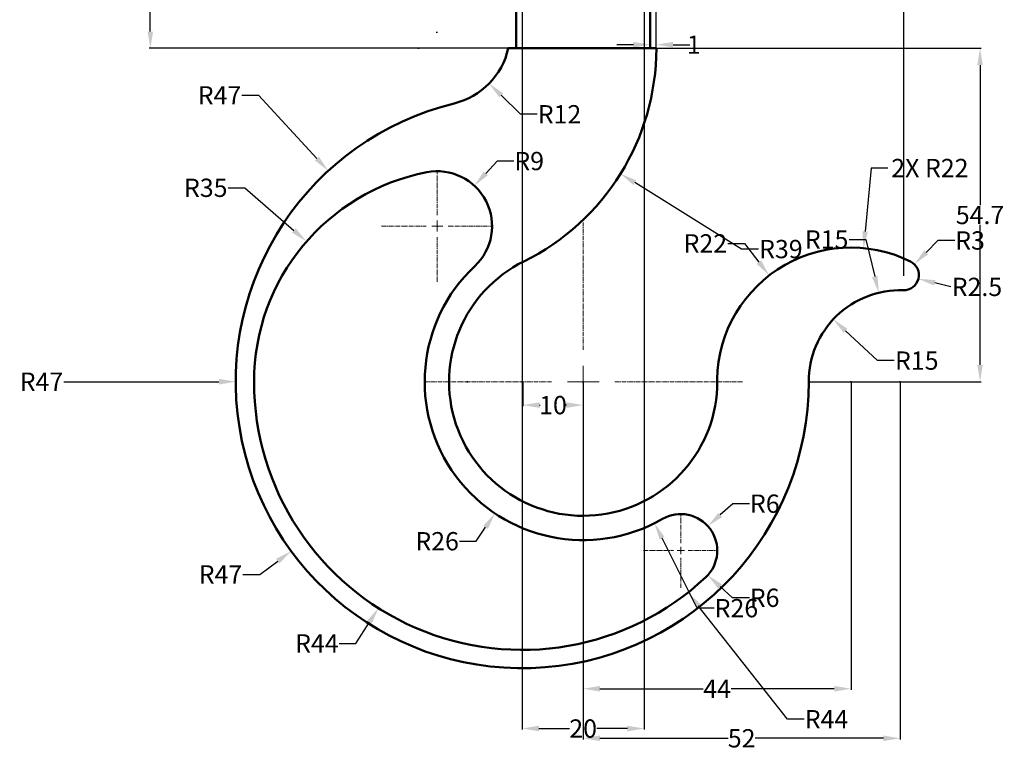
# Model space of a CAD drawing. Units: inches. Extents: x 7239 to 7401, y 3529 to 3727.
# Tile 1 of 2: x 7239 to 7400, y 3529 to 3648. Entities that reach past the tile are written whole.
import ezdxf

# ---------------------------------------------------------------- set-up
doc = ezdxf.new("R2010")
doc.units = ezdxf.units.IN
doc.header["$MEASUREMENT"] = 0
doc.linetypes.add('CENTER2', pattern=[1.125, 0.75, -0.125, 0.125, -0.125])
for name, color, linetype, lineweight in [('M-CNTR', 4, 'CENTER2', 18), ('M-DIMS', 2, 'Continuous', 25), ('M-OUTL', 7, 'Continuous', 50)]:
    doc.layers.add(name, color=color, linetype=linetype, lineweight=lineweight)
doc.styles.get("Standard").update_dxf_attribs({"font": 'arial.ttf'})
doc.dimstyles.get("Standard").update_dxf_attribs({"dimtxt": 3, "dimasz": 2.75, "dimexe": 0.18, "dimexo": 0.0625, "dimgap": 0.09, "dimtad": 0, "dimtih": 1, "dimtoh": 1, "dimdec": 0, "dimzin": 0, "dimdsep": 46, "dimtxsty": 'Standard', "dimcen": 0.09, "dimadec": 0, "dimazin": 0, "dimtfac": 1, "dimtdec": 0, "dimtofl": 0, "dimtmove": 0, "dimatfit": 3, "dimfxl": 1, "dimtolj": 1, "dimtzin": 0, "dimarcsym": 0})

# ---------------------------------------------------------------- blocks, each defined once
blk = doc.blocks.new('*U1')
at = {"layer": 'M-CNTR', "color": 0, "transparency": 16777216}
for p, q in [((0, 5.2), (0, 26.12)), ((-26.12, 0), (-5.2, 0)), ((5.2, 0), (26.12, 0)), ((0, -26.12), (0, -5.2))]:
    blk.add_line(p, q, dxfattribs=at)
at = {"layer": 'M-CNTR', "color": 0, "linetype": 'Continuous', "transparency": 16777216}
for p, q in [((0, -2.6), (0, 2.6)), ((-2.6, 0), (2.6, 0))]:
    blk.add_line(p, q, dxfattribs=at)
blk = doc.blocks.new('*U5')
at = {"layer": 'M-CNTR', "color": 0, "transparency": 16777216}
for p, q in [((0, 1.2), (0, 6.12)), ((-6.12, 0), (-1.2, 0)), ((1.2, 0), (6.12, 0)), ((0, -6.12), (0, -1.2))]:
    blk.add_line(p, q, dxfattribs=at)
at = {"layer": 'M-CNTR', "color": 0, "linetype": 'Continuous', "transparency": 16777216}
for p, q in [((-0.6, 0), (0.6, 0)), ((0, -0.6), (0, 0.6))]:
    blk.add_line(p, q, dxfattribs=at)
blk = doc.blocks.new('*U6')
at = {"layer": 'M-CNTR', "color": 0, "transparency": 16777216}
for p, q in [((0, 1.8), (0, 9.12)), ((-9.12, 0), (-1.8, 0)), ((1.8, 0), (9.12, 0)), ((0, -9.12), (0, -1.8))]:
    blk.add_line(p, q, dxfattribs=at)
at = {"layer": 'M-CNTR', "color": 0, "linetype": 'Continuous', "transparency": 16777216}
for p, q in [((-0.9, 0), (0.9, 0)), ((0, -0.9), (0, 0.9))]:
    blk.add_line(p, q, dxfattribs=at)
blk = doc.blocks.new('*D7')
at = {"layer": 'Defpoints', "color": 0, "transparency": 16777216}
for p in [(7289.29, 3623.58), (7321.11, 3589)]:
    blk.add_point(p, dxfattribs=at)
at = {"layer": 'M-DIMS', "color": 0, "lineweight": -2, "transparency": 16777216}
for p, q in [((7275.12, 3635.98), (7277.87, 3635.98)), ((7277.87, 3635.98), (7287.42, 3625.61)), ((7321.02, 3589), (7321.2, 3589)), ((7321.11, 3588.91), (7321.11, 3589.09))]:
    blk.add_line(p, q, dxfattribs=at)
at = {"layer": 'M-DIMS', "color": 0, "transparency": 16777216}
blk.add_solid([(7287.76, 3625.92), (7287.09, 3625.3), (7289.29, 3623.58)], dxfattribs=at)
at = {"layer": 'M-DIMS', "color": 0, "transparency": 16777216, "insert": (7271.45, 3635.98), "char_height": 3, "attachment_point": 5}
blk.add_mtext('\\A1;R47', dxfattribs=at)
blk = doc.blocks.new('*D8')
at = {"layer": 'Defpoints', "color": 0, "transparency": 16777216}
for p in [(7385.45, 3608.27), (7383.69, 3606.49)]:
    blk.add_point(p, dxfattribs=at)
at = {"layer": 'M-DIMS', "color": 0, "lineweight": -2, "transparency": 16777216}
for p, q in [((7389.32, 3612.17), (7387.38, 3610.22)), ((7392.07, 3612.17), (7389.32, 3612.17)), ((7383.6, 3606.49), (7383.78, 3606.49)), ((7383.69, 3606.4), (7383.69, 3606.58))]:
    blk.add_line(p, q, dxfattribs=at)
at = {"layer": 'M-DIMS', "color": 0, "transparency": 16777216}
blk.add_solid([(7387.06, 3610.54), (7387.71, 3609.9), (7385.45, 3608.27)], dxfattribs=at)
at = {"layer": 'M-DIMS', "color": 0, "transparency": 16777216, "insert": (7394.58, 3612.17), "char_height": 3, "attachment_point": 5}
blk.add_mtext('\\A1;R3', dxfattribs=at)
blk = doc.blocks.new('*D9')
at = {"layer": 'Defpoints', "color": 0, "transparency": 16777216}
for p in [(7372.14, 3599.23), (7383.11, 3589)]:
    blk.add_point(p, dxfattribs=at)
at = {"layer": 'M-DIMS', "color": 0, "lineweight": -2, "transparency": 16777216}
for p, q in [((7379.4, 3592.46), (7374.16, 3597.36)), ((7382.15, 3592.46), (7379.4, 3592.46))]:
    blk.add_line(p, q, dxfattribs=at)
at = {"layer": 'M-DIMS', "color": 0, "transparency": 16777216}
blk.add_solid([(7374.47, 3597.69), (7373.84, 3597.02), (7372.14, 3599.23)], dxfattribs=at)
at = {"layer": 'M-DIMS', "color": 0, "transparency": 16777216, "insert": (7385.84, 3592.46), "char_height": 3, "attachment_point": 5}
blk.add_mtext('\\A1;R15', dxfattribs=at)
blk = doc.blocks.new('*D10')
at = {"layer": 'Defpoints', "color": 0, "transparency": 16777216}
for p in [(7361.63, 3606.42), (7375.06, 3589)]:
    blk.add_point(p, dxfattribs=at)
at = {"layer": 'M-DIMS', "color": 0, "lineweight": -2, "transparency": 16777216}
for p, q in [((7354.82, 3611.69), (7357.57, 3611.69)), ((7357.57, 3611.69), (7359.95, 3608.6)), ((7374.97, 3589), (7375.15, 3589)), ((7375.06, 3588.91), (7375.06, 3589.09))]:
    blk.add_line(p, q, dxfattribs=at)
at = {"layer": 'M-DIMS', "color": 0, "transparency": 16777216}
blk.add_solid([(7360.31, 3608.88), (7359.59, 3608.32), (7361.63, 3606.42)], dxfattribs=at)
at = {"layer": 'M-DIMS', "color": 0, "transparency": 16777216, "insert": (7351.16, 3611.69), "char_height": 3, "attachment_point": 5}
blk.add_mtext('\\A1;R22', dxfattribs=at)
blk = doc.blocks.new('*D11')
at = {"layer": 'Defpoints', "color": 0, "transparency": 16777216}
for p in [(7351.57, 3565.31), (7347.11, 3561.29)]:
    blk.add_point(p, dxfattribs=at)
at = {"layer": 'M-DIMS', "color": 0, "lineweight": -2, "transparency": 16777216}
for p, q in [((7355.65, 3568.99), (7353.61, 3567.15)), ((7358.4, 3568.99), (7355.65, 3568.99)), ((7347.02, 3561.29), (7347.2, 3561.29)), ((7347.11, 3561.2), (7347.11, 3561.38))]:
    blk.add_line(p, q, dxfattribs=at)
at = {"layer": 'M-DIMS', "color": 0, "transparency": 16777216}
blk.add_solid([(7353.3, 3567.49), (7353.92, 3566.81), (7351.57, 3565.31)], dxfattribs=at)
at = {"layer": 'M-DIMS', "color": 0, "transparency": 16777216, "insert": (7360.91, 3568.99), "char_height": 3, "attachment_point": 5}
blk.add_mtext('\\A1;R6', dxfattribs=at)
blk = doc.blocks.new('*D12')
at = {"layer": 'Defpoints', "color": 0, "transparency": 16777216}
for p in [(7321.11, 3589), (7283.22, 3561.19)]:
    blk.add_point(p, dxfattribs=at)
at = {"layer": 'M-DIMS', "color": 0, "lineweight": -2, "transparency": 16777216}
for p, q in [((7321.02, 3589), (7321.2, 3589)), ((7321.11, 3588.91), (7321.11, 3589.09)), ((7278.04, 3557.39), (7281.01, 3559.57)), ((7275.29, 3557.39), (7278.04, 3557.39))]:
    blk.add_line(p, q, dxfattribs=at)
at = {"layer": 'M-DIMS', "color": 0, "transparency": 16777216}
blk.add_solid([(7280.74, 3559.94), (7281.28, 3559.2), (7283.22, 3561.19)], dxfattribs=at)
at = {"layer": 'M-DIMS', "color": 0, "transparency": 16777216, "insert": (7271.61, 3557.39), "char_height": 3, "attachment_point": 5}
blk.add_mtext('\\A1;R47', dxfattribs=at)
blk = doc.blocks.new('*D13')
at = {"layer": 'Defpoints', "color": 0, "transparency": 16777216}
for p in [(7321.11, 3589), (7297.52, 3551.86)]:
    blk.add_point(p, dxfattribs=at)
at = {"layer": 'M-DIMS', "color": 0, "lineweight": -2, "transparency": 16777216}
for p, q in [((7321.02, 3589), (7321.2, 3589)), ((7321.11, 3588.91), (7321.11, 3589.09)), ((7293.84, 3546.07), (7296.04, 3549.54)), ((7291.09, 3546.07), (7293.84, 3546.07))]:
    blk.add_line(p, q, dxfattribs=at)
at = {"layer": 'M-DIMS', "color": 0, "transparency": 16777216}
blk.add_solid([(7295.66, 3549.79), (7296.43, 3549.3), (7297.52, 3551.86)], dxfattribs=at)
at = {"layer": 'M-DIMS', "color": 0, "transparency": 16777216, "insert": (7287.42, 3546.07), "char_height": 3, "attachment_point": 5}
blk.add_mtext('\\A1;R44', dxfattribs=at)
blk = doc.blocks.new('*D14')
at = {"layer": 'Defpoints', "color": 0, "transparency": 16777216}
for p in [(7313.26, 3621.15), (7307.17, 3614.53)]:
    blk.add_point(p, dxfattribs=at)
at = {"layer": 'M-DIMS', "color": 0, "lineweight": -2, "transparency": 16777216}
for p, q in [((7316.99, 3625.2), (7315.12, 3623.17)), ((7319.74, 3625.2), (7316.99, 3625.2)), ((7307.08, 3614.53), (7307.26, 3614.53)), ((7307.17, 3614.44), (7307.17, 3614.62))]:
    blk.add_line(p, q, dxfattribs=at)
at = {"layer": 'M-DIMS', "color": 0, "transparency": 16777216}
blk.add_solid([(7314.79, 3623.48), (7315.46, 3622.86), (7313.26, 3621.15)], dxfattribs=at)
at = {"layer": 'M-DIMS', "color": 0, "transparency": 16777216, "insert": (7322.25, 3625.2), "char_height": 3, "attachment_point": 5}
blk.add_mtext('\\A1;R9', dxfattribs=at)
blk = doc.blocks.new('*D15')
at = {"layer": 'Defpoints', "color": 0, "transparency": 16777216}
for p in [(7331.11, 3589), (7316.64, 3567.4)]:
    blk.add_point(p, dxfattribs=at)
at = {"layer": 'M-DIMS', "color": 0, "lineweight": -2, "transparency": 16777216}
for p, q in [((7331.02, 3589), (7331.2, 3589)), ((7331.11, 3588.91), (7331.11, 3589.09)), ((7313.58, 3562.83), (7315.11, 3565.12)), ((7310.83, 3562.83), (7313.58, 3562.83))]:
    blk.add_line(p, q, dxfattribs=at)
at = {"layer": 'M-DIMS', "color": 0, "transparency": 16777216}
blk.add_solid([(7314.73, 3565.37), (7315.49, 3564.86), (7316.64, 3567.4)], dxfattribs=at)
at = {"layer": 'M-DIMS', "color": 0, "transparency": 16777216, "insert": (7307.15, 3562.83), "char_height": 3, "attachment_point": 5}
blk.add_mtext('\\A1;R26', dxfattribs=at)
blk = doc.blocks.new('*D16')
at = {"layer": 'Defpoints', "color": 0, "transparency": 16777216}
for p in [(7331.11, 3588.91), (7383.11, 3589), (7383.11, 3530.5)]:
    blk.add_point(p, dxfattribs=at)
at = {"layer": 'M-DIMS', "color": 0, "lineweight": -2, "transparency": 16777216}
for p, q in [((7331.11, 3588.85), (7331.11, 3530.32)), ((7383.11, 3588.94), (7383.11, 3530.32)), ((7333.86, 3530.5), (7354.89, 3530.5)), ((7380.36, 3530.5), (7359.34, 3530.5))]:
    blk.add_line(p, q, dxfattribs=at)
at = {"layer": 'M-DIMS', "color": 0, "transparency": 16777216}
for points in [[(7333.86, 3530.96), (7333.86, 3530.04), (7331.11, 3530.5)], [(7380.36, 3530.96), (7380.36, 3530.04), (7383.11, 3530.5)]]:
    blk.add_solid(points, dxfattribs=at)
at = {"layer": 'M-DIMS', "color": 0, "transparency": 16777216, "insert": (7357.11, 3530.5), "char_height": 3, "attachment_point": 5}
blk.add_mtext('\\A1;52', dxfattribs=at)
blk = doc.blocks.new('*D17')
at = {"layer": 'Defpoints', "color": 0, "transparency": 16777216}
for p in [(7331.11, 3588.91), (7375.06, 3588.91), (7375.06, 3538.63)]:
    blk.add_point(p, dxfattribs=at)
at = {"layer": 'M-DIMS', "color": 0, "lineweight": -2, "transparency": 16777216}
for p, q in [((7331.11, 3588.85), (7331.11, 3538.45)), ((7375.06, 3588.85), (7375.06, 3538.45)), ((7333.86, 3538.63), (7350.8, 3538.63)), ((7372.31, 3538.63), (7355.38, 3538.63))]:
    blk.add_line(p, q, dxfattribs=at)
at = {"layer": 'M-DIMS', "color": 0, "transparency": 16777216}
for points in [[(7333.86, 3539.09), (7333.86, 3538.17), (7331.11, 3538.63)], [(7372.31, 3539.09), (7372.31, 3538.17), (7375.06, 3538.63)]]:
    blk.add_solid(points, dxfattribs=at)
at = {"layer": 'M-DIMS', "color": 0, "transparency": 16777216, "insert": (7353.09, 3538.63), "char_height": 3, "attachment_point": 5}
blk.add_mtext('\\A1;44', dxfattribs=at)
blk = doc.blocks.new('*D18')
at = {"layer": 'Defpoints', "color": 0, "transparency": 16777216}
for p in [(7321.2, 3589), (7331.11, 3589.09), (7321.2, 3585.16)]:
    blk.add_point(p, dxfattribs=at)
at = {"layer": 'M-DIMS', "color": 0, "lineweight": -2, "transparency": 16777216}
for p, q in [((7321.2, 3588.94), (7321.2, 3584.98)), ((7331.11, 3589.03), (7331.11, 3584.98)), ((7323.95, 3585.16), (7324.07, 3585.16)), ((7328.36, 3585.16), (7328.25, 3585.16))]:
    blk.add_line(p, q, dxfattribs=at)
at = {"layer": 'M-DIMS', "color": 0, "transparency": 16777216}
for points in [[(7323.95, 3585.62), (7323.95, 3584.7), (7321.2, 3585.16)], [(7328.36, 3585.62), (7328.36, 3584.7), (7331.11, 3585.16)]]:
    blk.add_solid(points, dxfattribs=at)
at = {"layer": 'M-DIMS', "color": 0, "transparency": 16777216, "insert": (7326.16, 3585.16), "char_height": 3, "attachment_point": 5}
blk.add_mtext('\\A1;10', dxfattribs=at)
blk = doc.blocks.new('*D19')
at = {"layer": 'Defpoints', "color": 0, "transparency": 16777216}
for p in [(7285.73, 3612), (7312.11, 3589)]:
    blk.add_point(p, dxfattribs=at)
at = {"layer": 'M-DIMS', "color": 0, "lineweight": -2, "transparency": 16777216}
for p, q in [((7272.88, 3620.81), (7275.63, 3620.81)), ((7275.63, 3620.81), (7283.66, 3613.81)), ((7312.02, 3589), (7312.2, 3589)), ((7312.11, 3588.91), (7312.11, 3589.09))]:
    blk.add_line(p, q, dxfattribs=at)
at = {"layer": 'M-DIMS', "color": 0, "transparency": 16777216}
blk.add_solid([(7283.96, 3614.15), (7283.36, 3613.46), (7285.73, 3612)], dxfattribs=at)
at = {"layer": 'M-DIMS', "color": 0, "transparency": 16777216, "insert": (7269.19, 3620.81), "char_height": 3, "attachment_point": 5}
blk.add_mtext('\\A1;R35', dxfattribs=at)
blk = doc.blocks.new('*D20')
at = {"layer": 'Defpoints', "color": 0, "transparency": 16777216}
for p in [(7343.11, 3644.29), (7342.11, 3643.7), (7343.11, 3643.7)]:
    blk.add_point(p, dxfattribs=at)
at = {"layer": 'M-DIMS', "color": 0, "lineweight": -2, "transparency": 16777216}
for p, q in [((7339.36, 3644.29), (7336.61, 3644.29)), ((7342.11, 3643.76), (7342.11, 3644.47)), ((7343.11, 3643.76), (7343.11, 3644.47)), ((7345.86, 3644.29), (7348.61, 3644.29))]:
    blk.add_line(p, q, dxfattribs=at)
at = {"layer": 'M-DIMS', "color": 0, "transparency": 16777216}
for points in [[(7339.36, 3644.74), (7339.36, 3643.83), (7342.11, 3644.29)], [(7345.86, 3644.74), (7345.86, 3643.83), (7343.11, 3644.29)]]:
    blk.add_solid(points, dxfattribs=at)
at = {"layer": 'M-DIMS', "color": 0, "transparency": 16777216, "insert": (7349.26, 3644.29), "char_height": 3, "attachment_point": 5}
blk.add_mtext('\\A1;1', dxfattribs=at)
blk = doc.blocks.new('*D22')
at = {"layer": 'Defpoints', "color": 0, "transparency": 16777216}
for p in [(7260.1, 3668.7), (7320.11, 3668.7), (7320.11, 3643.7)]:
    blk.add_point(p, dxfattribs=at)
at = {"layer": 'M-DIMS', "color": 0, "lineweight": -2, "transparency": 16777216}
for p, q in [((7320.05, 3668.7), (7259.92, 3668.7)), ((7260.1, 3665.95), (7260.1, 3657.82)), ((7260.1, 3646.45), (7260.1, 3654.58)), ((7320.05, 3643.7), (7259.92, 3643.7))]:
    blk.add_line(p, q, dxfattribs=at)
at = {"layer": 'M-DIMS', "color": 0, "transparency": 16777216}
for points in [[(7259.64, 3665.95), (7260.56, 3665.95), (7260.1, 3668.7)], [(7259.64, 3646.45), (7260.56, 3646.45), (7260.1, 3643.7)]]:
    blk.add_solid(points, dxfattribs=at)
at = {"layer": 'M-DIMS', "color": 0, "transparency": 16777216, "insert": (7260.1, 3656.2), "char_height": 3, "attachment_point": 5}
blk.add_mtext('\\A1;25', dxfattribs=at)
blk = doc.blocks.new('*D32')
at = {"layer": 'Defpoints', "color": 0, "transparency": 16777216}
for p in [(7343.11, 3643.7), (7396.22, 3643.7), (7368.11, 3589)]:
    blk.add_point(p, dxfattribs=at)
at = {"layer": 'M-DIMS', "color": 0, "lineweight": -2, "transparency": 16777216}
for p, q in [((7343.18, 3643.7), (7396.4, 3643.7)), ((7396.22, 3640.95), (7396.22, 3617.97)), ((7396.22, 3591.75), (7396.22, 3614.74)), ((7368.18, 3589), (7396.4, 3589))]:
    blk.add_line(p, q, dxfattribs=at)
at = {"layer": 'M-DIMS', "color": 0, "transparency": 16777216}
for points in [[(7395.77, 3640.95), (7396.68, 3640.95), (7396.22, 3643.7)], [(7395.77, 3591.75), (7396.68, 3591.75), (7396.22, 3589)]]:
    blk.add_solid(points, dxfattribs=at)
at = {"layer": 'M-DIMS', "color": 0, "transparency": 16777216, "insert": (7396.22, 3616.35), "char_height": 3, "attachment_point": 5}
blk.add_mtext('\\A1;54.7', dxfattribs=at)
blk = doc.blocks.new('*D33')
at = {"layer": 'Defpoints', "color": 0, "transparency": 16777216}
for p in [(7321.11, 3672.7), (7341.11, 3672.7), (7341.11, 3532.1)]:
    blk.add_point(p, dxfattribs=at)
at = {"layer": 'M-DIMS', "color": 0, "lineweight": -2, "transparency": 16777216}
for p, q in [((7321.11, 3672.64), (7321.11, 3531.92)), ((7341.11, 3672.64), (7341.11, 3531.92)), ((7323.86, 3532.1), (7328.85, 3532.1)), ((7338.36, 3532.1), (7333.37, 3532.1))]:
    blk.add_line(p, q, dxfattribs=at)
at = {"layer": 'M-DIMS', "color": 0, "transparency": 16777216}
for points in [[(7323.86, 3532.56), (7323.86, 3531.64), (7321.11, 3532.1)], [(7338.36, 3532.56), (7338.36, 3531.64), (7341.11, 3532.1)]]:
    blk.add_solid(points, dxfattribs=at)
at = {"layer": 'M-DIMS', "color": 0, "transparency": 16777216, "insert": (7331.11, 3532.1), "char_height": 3, "attachment_point": 5}
blk.add_mtext('\\A1;20', dxfattribs=at)
blk = doc.blocks.new('*D35')
at = {"layer": 'Defpoints', "color": 0, "transparency": 16777216}
for p in [(7383.69, 3723.87), (7343.11, 3643.7), (7383.69, 3606.49)]:
    blk.add_point(p, dxfattribs=at)
at = {"layer": 'M-DIMS', "color": 0, "lineweight": -2, "transparency": 16777216}
for p, q in [((7343.11, 3643.76), (7343.11, 3724.05)), ((7345.86, 3723.87), (7358.19, 3723.87)), ((7380.94, 3723.87), (7368.61, 3723.87)), ((7383.69, 3606.55), (7383.69, 3724.05))]:
    blk.add_line(p, q, dxfattribs=at)
at = {"layer": 'M-DIMS', "color": 0, "transparency": 16777216}
for points in [[(7345.86, 3724.33), (7345.86, 3723.41), (7343.11, 3723.87)], [(7380.94, 3724.33), (7380.94, 3723.41), (7383.69, 3723.87)]]:
    blk.add_solid(points, dxfattribs=at)
at = {"layer": 'M-DIMS', "color": 0, "transparency": 16777216, "insert": (7363.4, 3723.87), "char_height": 3, "attachment_point": 5}
blk.add_mtext('\\A1;40.57', dxfattribs=at)
blk = doc.blocks.new('*D36')
at = {"layer": 'Defpoints', "color": 0, "transparency": 16777216}
for p in [(7274.11, 3589), (7321.11, 3589)]:
    blk.add_point(p, dxfattribs=at)
at = {"layer": 'M-DIMS', "color": 0, "lineweight": -2, "transparency": 16777216}
for p, q in [((7245.91, 3589), (7271.36, 3589)), ((7321.02, 3589), (7321.2, 3589)), ((7321.11, 3588.91), (7321.11, 3589.09))]:
    blk.add_line(p, q, dxfattribs=at)
at = {"layer": 'M-DIMS', "color": 0, "transparency": 16777216}
blk.add_solid([(7271.36, 3589.46), (7271.36, 3588.54), (7274.11, 3589)], dxfattribs=at)
at = {"layer": 'M-DIMS', "color": 0, "transparency": 16777216, "insert": (7242.24, 3589), "char_height": 3, "attachment_point": 5}
blk.add_mtext('\\A1;R47', dxfattribs=at)
blk = doc.blocks.new('*D37')
at = {"layer": 'Defpoints', "color": 0, "transparency": 16777216}
for p in [(7321.11, 3589), (7348.3, 3554.4)]:
    blk.add_point(p, dxfattribs=at)
at = {"layer": 'M-DIMS', "color": 0, "lineweight": -2, "transparency": 16777216}
for p, q in [((7321.02, 3589), (7321.2, 3589)), ((7321.11, 3588.91), (7321.11, 3589.09)), ((7364.61, 3533.64), (7350, 3552.24)), ((7367.36, 3533.64), (7364.61, 3533.64))]:
    blk.add_line(p, q, dxfattribs=at)
at = {"layer": 'M-DIMS', "color": 0, "transparency": 16777216}
blk.add_solid([(7350.36, 3552.52), (7349.64, 3551.96), (7348.3, 3554.4)], dxfattribs=at)
at = {"layer": 'M-DIMS', "color": 0, "transparency": 16777216, "insert": (7371.03, 3533.64), "char_height": 3, "attachment_point": 5}
blk.add_mtext('\\A1;R44', dxfattribs=at)
blk = doc.blocks.new('*D38')
at = {"layer": 'Defpoints', "color": 0, "transparency": 16777216}
for p in [(7304.11, 3643.7), (7337.24, 3623.11)]:
    blk.add_point(p, dxfattribs=at)
at = {"layer": 'M-DIMS', "color": 0, "lineweight": -2, "transparency": 16777216}
for p, q in [((7304.02, 3643.7), (7304.2, 3643.7)), ((7304.11, 3643.61), (7304.11, 3643.79)), ((7357.11, 3610.76), (7339.57, 3621.66)), ((7359.86, 3610.76), (7357.11, 3610.76))]:
    blk.add_line(p, q, dxfattribs=at)
at = {"layer": 'M-DIMS', "color": 0, "transparency": 16777216}
blk.add_solid([(7339.81, 3622.05), (7339.33, 3621.27), (7337.24, 3623.11)], dxfattribs=at)
at = {"layer": 'M-DIMS', "color": 0, "transparency": 16777216, "insert": (7363.54, 3610.76), "char_height": 3, "attachment_point": 5}
blk.add_mtext('\\A1;R39', dxfattribs=at)
blk = doc.blocks.new('*D39')
at = {"layer": 'Defpoints', "color": 0, "transparency": 16777216}
for p in [(7331.11, 3589), (7342.81, 3565.78)]:
    blk.add_point(p, dxfattribs=at)
at = {"layer": 'M-DIMS', "color": 0, "lineweight": -2, "transparency": 16777216}
for p, q in [((7331.02, 3589), (7331.2, 3589)), ((7331.11, 3588.91), (7331.11, 3589.09)), ((7349.83, 3551.85), (7344.05, 3563.32)), ((7352.58, 3551.85), (7349.83, 3551.85))]:
    blk.add_line(p, q, dxfattribs=at)
at = {"layer": 'M-DIMS', "color": 0, "transparency": 16777216}
blk.add_solid([(7344.46, 3563.53), (7343.64, 3563.12), (7342.81, 3565.78)], dxfattribs=at)
at = {"layer": 'M-DIMS', "color": 0, "transparency": 16777216, "insert": (7356.25, 3551.85), "char_height": 3, "attachment_point": 5}
blk.add_mtext('\\A1;R26', dxfattribs=at)
blk = doc.blocks.new('*D40')
at = {"layer": 'Defpoints', "color": 0, "transparency": 16777216}
for p in [(7377.11, 3610.91), (7375.06, 3589)]:
    blk.add_point(p, dxfattribs=at)
at = {"layer": 'M-DIMS', "color": 0, "lineweight": -2, "transparency": 16777216}
for p, q in [((7378.34, 3624.05), (7377.37, 3613.64)), ((7381.09, 3624.05), (7378.34, 3624.05)), ((7374.97, 3589), (7375.15, 3589)), ((7375.06, 3588.91), (7375.06, 3589.09))]:
    blk.add_line(p, q, dxfattribs=at)
at = {"layer": 'M-DIMS', "color": 0, "transparency": 16777216}
blk.add_solid([(7376.91, 3613.69), (7377.82, 3613.6), (7377.11, 3610.91)], dxfattribs=at)
at = {"layer": 'M-DIMS', "color": 0, "transparency": 16777216, "insert": (7387.99, 3624.05), "char_height": 3, "attachment_point": 5}
blk.add_mtext('\\A1;2X R22', dxfattribs=at)
blk = doc.blocks.new('*D41')
at = {"layer": 'Defpoints', "color": 0, "transparency": 16777216}
for p in [(7379.6, 3603.58), (7383.11, 3589)]:
    blk.add_point(p, dxfattribs=at)
at = {"layer": 'M-DIMS', "color": 0, "lineweight": -2, "transparency": 16777216}
for p, q in [((7374.74, 3612.33), (7377.49, 3612.33)), ((7377.49, 3612.33), (7378.95, 3606.26)), ((7383.02, 3589), (7383.2, 3589)), ((7383.11, 3588.91), (7383.11, 3589.09))]:
    blk.add_line(p, q, dxfattribs=at)
at = {"layer": 'M-DIMS', "color": 0, "transparency": 16777216}
blk.add_solid([(7379.4, 3606.36), (7378.51, 3606.15), (7379.6, 3603.58)], dxfattribs=at)
at = {"layer": 'M-DIMS', "color": 0, "transparency": 16777216, "insert": (7371.05, 3612.33), "char_height": 3, "attachment_point": 5}
blk.add_mtext('\\A1;R15', dxfattribs=at)
blk = doc.blocks.new('*D42')
at = {"layer": 'Defpoints', "color": 0, "transparency": 16777216}
for p in [(7307.11, 3646.32), (7315.68, 3637.92)]:
    blk.add_point(p, dxfattribs=at)
at = {"layer": 'M-DIMS', "color": 0, "lineweight": -2, "transparency": 16777216}
for p, q in [((7307.02, 3646.32), (7307.2, 3646.32)), ((7307.11, 3646.23), (7307.11, 3646.41)), ((7320.82, 3632.87), (7317.65, 3635.99)), ((7323.57, 3632.87), (7320.82, 3632.87))]:
    blk.add_line(p, q, dxfattribs=at)
at = {"layer": 'M-DIMS', "color": 0, "transparency": 16777216}
blk.add_solid([(7317.97, 3636.32), (7317.33, 3635.66), (7315.68, 3637.92)], dxfattribs=at)
at = {"layer": 'M-DIMS', "color": 0, "transparency": 16777216, "insert": (7327.23, 3632.87), "char_height": 3, "attachment_point": 5}
blk.add_mtext('\\A1;R12', dxfattribs=at)
blk = doc.blocks.new('*D43')
at = {"layer": 'Defpoints', "color": 0, "transparency": 16777216}
for p in [(7347.11, 3561.29), (7351.55, 3557.25)]:
    blk.add_point(p, dxfattribs=at)
at = {"layer": 'M-DIMS', "color": 0, "lineweight": -2, "transparency": 16777216}
for p, q in [((7347.02, 3561.29), (7347.2, 3561.29)), ((7347.11, 3561.2), (7347.11, 3561.38)), ((7355.62, 3553.55), (7353.58, 3555.4)), ((7358.37, 3553.55), (7355.62, 3553.55))]:
    blk.add_line(p, q, dxfattribs=at)
at = {"layer": 'M-DIMS', "color": 0, "transparency": 16777216}
blk.add_solid([(7353.89, 3555.74), (7353.28, 3555.06), (7351.55, 3557.25)], dxfattribs=at)
at = {"layer": 'M-DIMS', "color": 0, "transparency": 16777216, "insert": (7360.88, 3553.55), "char_height": 3, "attachment_point": 5}
blk.add_mtext('\\A1;R6', dxfattribs=at)
blk = doc.blocks.new('*D45')
at = {"layer": 'Defpoints', "color": 0, "transparency": 16777216}
for p in [(7383.69, 3606.49), (7386.11, 3605.88)]:
    blk.add_point(p, dxfattribs=at)
at = {"layer": 'M-DIMS', "color": 0, "lineweight": -2, "transparency": 16777216}
for p, q in [((7383.6, 3606.49), (7383.78, 3606.49)), ((7383.69, 3606.4), (7383.69, 3606.58)), ((7391.45, 3604.55), (7388.78, 3605.22))]:
    blk.add_line(p, q, dxfattribs=at)
at = {"layer": 'M-DIMS', "color": 0, "transparency": 16777216}
blk.add_solid([(7388.89, 3605.66), (7388.67, 3604.77), (7386.11, 3605.88)], dxfattribs=at)
at = {"layer": 'M-DIMS', "color": 0, "transparency": 16777216, "insert": (7395.71, 3604.55), "char_height": 3, "attachment_point": 5}
blk.add_mtext('\\A1;R2.5', dxfattribs=at)

msp = doc.modelspace()

# ---------------------------------------------------------------- linework, layer by layer
at = {"layer": 'M-OUTL'}
for p, q in [((7320.114, 3643.7), (7320.114, 3668.7)), ((7342.114, 3668.7), (7342.114, 3643.7)), ((7319.114, 3643.7), (7318.825, 3643.7)), ((7321.114, 3643.7), (7319.114, 3643.7)), ((7343.114, 3643.7), (7321.114, 3643.7)), ((7353.064, 3589.001), (7353.114, 3589.001)), ((7353.064, 3589.001), (7353.114, 3589.001)), ((7353.114, 3589.001), (7353.064, 3589.001))]:
    msp.add_line(p, q, dxfattribs=at)
for centre, radius, start, end in [((7307.114, 3646.316), 12, 283.72654, 347.40967), ((7304.114, 3643.7), 39, 296.27136, 0), ((7321.114, 3589.001), 47, 103.72654, 0), ((7312.114, 3589.001), 35, 100.96932, 180), ((7307.167, 3614.526), 9, 313.17355, 100.96932), ((7375.064, 3589.001), 22, 63.76099, 182.73173), ((7331.114, 3589.001), 22, 116.27136, 2.73173), ((7383.685, 3606.492), 2.5, 268.12929, 63.76099), ((7331.114, 3589.001), 26, 133.17355, 300), ((7383.114, 3589.001), 15, 88.12929, 180), ((7321.114, 3589.001), 44, 179.99978, 313.17355), ((7347.114, 3561.288), 6, 313.17355, 120)]:
    msp.add_arc(centre, radius, start, end, dxfattribs=at)

# ---------------------------------------------------------------- block references
at = {"layer": 'M-CNTR'}
for name, p in [('*U6', (7307.167, 3614.526)), ('*U1', (7331.114, 3589.001)), ('*U5', (7347.114, 3561.288))]:
    msp.add_blockref(name, p, dxfattribs=at)

# ---------------------------------------------------------------- dimensions: what is measured, and where the dimension line sits
at = {"layer": 'M-DIMS'}
for base, p1, p2, override, picture, middle in [((7383.685, 3723.87), (7343.114, 3643.7), (7383.685, 3606.492), {"dimdec": 2, "dimlfac": 1, "dimrnd": 0, "dimzin": 0, "dimdsep": 46, "dimlunit": 2}, '*D35', (7363.4, 3723.87)), ((7341.114, 3532.101), (7321.114, 3672.7), (7341.114, 3672.7), {"dimdec": 0, "dimlfac": 1, "dimrnd": 0, "dimzin": 0, "dimdsep": 46, "dimlunit": 2}, '*D33', (7331.114, 3532.101)), ((7343.114, 3644.285), (7342.114, 3643.7), (7343.114, 3643.7), {"dimclrd": 0, "dimclre": 0, "dimclrt": 0}, '*D20', (7349.257, 3644.285)), ((7321.204, 3585.163), (7331.114, 3589.091), (7321.204, 3589.001), {"dimclrd": 0, "dimclre": 0, "dimclrt": 0}, '*D18', (7326.159, 3585.163)), ((7383.114, 3530.498), (7331.114, 3588.911), (7383.114, 3589.001), {"dimclrd": 0, "dimclre": 0, "dimclrt": 0}, '*D16', (7357.114, 3530.498)), ((7375.064, 3538.628), (7331.114, 3588.911), (7375.064, 3588.911), {"dimclrd": 0, "dimclre": 0, "dimclrt": 0}, '*D17', (7353.089, 3538.628))]:
    dim = msp.add_linear_dim(base=base, p1=p1, p2=p2, dimstyle='Standard', override=override, dxfattribs=at)
    dim.commit()
    dim.dimension.update_dxf_attribs({"geometry": picture, "text_midpoint": middle})
dim = msp.add_aligned_dim(p1=(7320.114, 3643.7), p2=(7320.114, 3668.7), distance=60.013, dimstyle='Standard', override={"dimclrd": 0, "dimclre": 0, "dimclrt": 0}, dxfattribs=at)
dim.commit()
dim.dimension.update_dxf_attribs({"geometry": '*D22', "text_midpoint": (7260.101, 3656.2)})
for center, mpoint, override, picture, middle in [((7307.114, 3646.316), (7315.683, 3637.915), {"dimdec": 0, "dimlfac": 1, "dimrnd": 0, "dimzin": 0, "dimdsep": 46, "dimlunit": 2}, '*D42', (7327.233, 3632.875)), ((7304.114, 3643.7), (7337.237, 3623.112), {"dimdec": 0, "dimlfac": 1, "dimrnd": 0, "dimzin": 0, "dimdsep": 46, "dimlunit": 2}, '*D38', (7363.538, 3610.759)), ((7321.114, 3589.001), (7289.286, 3623.584), {"dimclrd": 0, "dimclre": 0, "dimclrt": 0}, '*D7', (7271.449, 3635.985)), ((7312.114, 3589.001), (7285.733, 3612.002), {"dimclrd": 0, "dimclre": 0, "dimclrt": 0}, '*D19', (7269.192, 3620.813)), ((7375.064, 3589.001), (7361.631, 3606.424), {"dimclrd": 0, "dimclre": 0, "dimclrt": 0}, '*D10', (7351.159, 3611.693)), ((7383.114, 3589.001), (7379.599, 3603.583), {"dimdec": 0, "dimlfac": 1, "dimrnd": 0, "dimzin": 0, "dimdsep": 46, "dimlunit": 2}, '*D41', (7371.055, 3612.333)), ((7383.114, 3589.001), (7372.144, 3599.231), {"dimclrd": 0, "dimclre": 0, "dimclrt": 0}, '*D9', (7385.838, 3592.462)), ((7321.114, 3589.001), (7274.114, 3589), {"dimdec": 0, "dimlfac": 1, "dimrnd": 0, "dimzin": 0, "dimdsep": 46, "dimlunit": 2}, '*D36', (7245.914, 3588.999)), ((7321.114, 3589.001), (7283.224, 3561.193), {"dimclrd": 0, "dimclre": 0, "dimclrt": 0}, '*D12', (7271.612, 3557.385)), ((7321.114, 3589.001), (7297.517, 3551.864), {"dimclrd": 0, "dimclre": 0, "dimclrt": 0}, '*D13', (7287.42, 3546.073)), ((7321.114, 3589.001), (7348.298, 3554.403), {"dimdec": 0, "dimlfac": 1, "dimrnd": 0, "dimzin": 0, "dimdsep": 46, "dimlunit": 2}, '*D37', (7371.026, 3533.644)), ((7331.114, 3589.001), (7342.81, 3565.78), {"dimdec": 0, "dimlfac": 1, "dimrnd": 0, "dimzin": 0, "dimdsep": 46, "dimlunit": 2}, '*D39', (7356.251, 3551.848))]:
    dim = msp.add_radius_dim(center=center, mpoint=mpoint, dimstyle='Standard', override=override, dxfattribs=at)
    dim.commit()
    dim.dimension.update_dxf_attribs({"geometry": picture, "text_midpoint": middle, "dimtype": 164})
dim = msp.add_linear_dim(base=(7396.223, 3643.7), p1=(7368.114, 3589.001), p2=(7343.114, 3643.7), angle=90, dimstyle='Standard', override={"dimdec": 1, "dimlfac": 1, "dimrnd": 0, "dimzin": 0, "dimdsep": 46, "dimlunit": 2}, dxfattribs=at)
dim.commit()
dim.dimension.update_dxf_attribs({"geometry": '*D32', "text_midpoint": (7396.223, 3616.351)})
dim = msp.add_radius_dim(center=(7375.064, 3589.001), mpoint=(7377.11, 3610.906), text='2X <>', dimstyle='Standard', override={"dimdec": 0, "dimlfac": 1, "dimrnd": 0, "dimzin": 0, "dimdsep": 46, "dimlunit": 2}, dxfattribs=at)
dim.commit()
dim.dimension.update_dxf_attribs({"geometry": '*D40', "text_midpoint": (7387.995, 3624.049), "dimtype": 164})
for center, mpoint, override, picture, middle in [((7307.167, 3614.526), (7313.262, 3621.148), {"dimclrd": 0, "dimclre": 0, "dimclrt": 0}, '*D14', (7322.248, 3625.195)), ((7383.68532, 3606.49175), (7385.44558, 3608.26699), {"dimclrd": 0, "dimclre": 0, "dimclrt": 0}, '*D8', (7394.57698, 3612.17252)), ((7383.685, 3606.492), (7386.111, 3605.885), {"dimdec": 1, "dimlfac": 1, "dimrnd": 0, "dimzin": 0, "dimdsep": 46, "dimlunit": 2}, '*D45', (7395.714, 3604.55)), ((7331.114, 3589.001), (7316.64, 3567.402), {"dimclrd": 0, "dimclre": 0, "dimclrt": 0}, '*D15', (7307.155, 3562.834)), ((7347.114, 3561.288), (7351.568, 3565.308), {"dimclrd": 0, "dimclre": 0, "dimclrt": 0}, '*D11', (7360.909, 3568.993)), ((7347.114, 3561.288), (7351.551, 3557.25), {"dimdec": 0, "dimlfac": 1, "dimrnd": 0, "dimzin": 0, "dimdsep": 46, "dimlunit": 2}, '*D43', (7360.876, 3553.547))]:
    dim = msp.add_radius_dim(center=center, mpoint=mpoint, dimstyle='Standard', override=override, dxfattribs=at)
    dim.commit()
    dim.dimension.update_dxf_attribs({"geometry": picture, "text_midpoint": middle})

doc.saveas('drawing.dxf')
